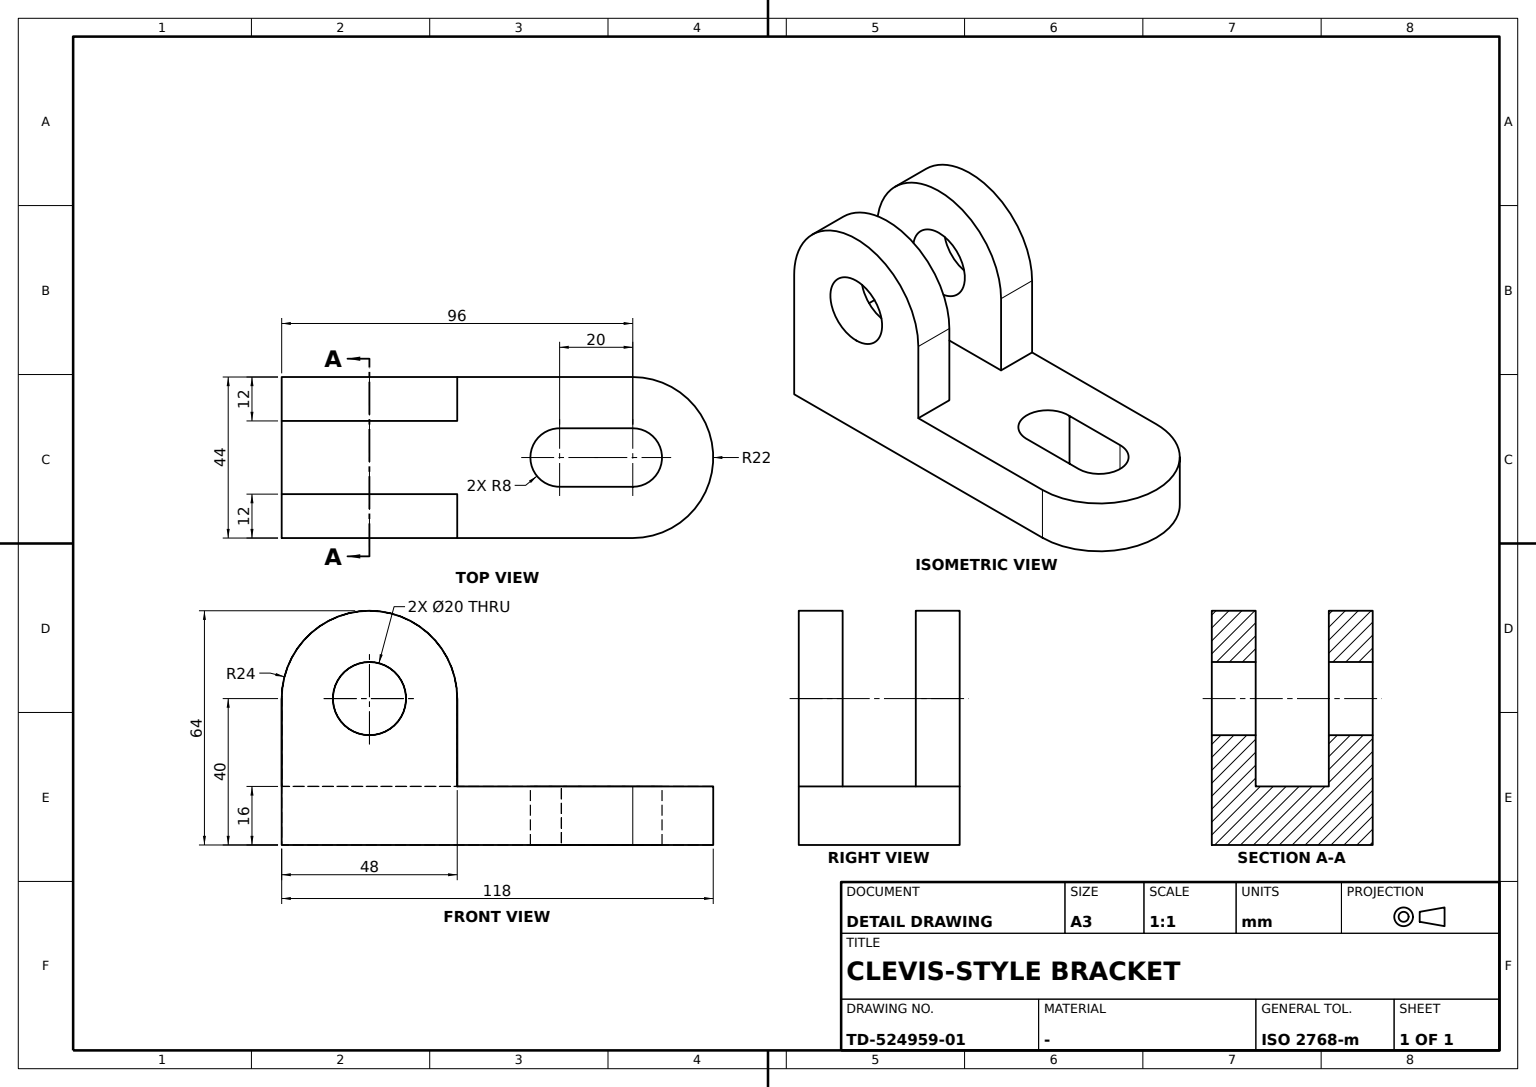
CATIA V5 part; units mm, degrees
sketch "Sketch1" plane through (0, 0, 0) normal (0, 0, 1) x (1, 0, 0)
  line L0 (-48, 22) -> (-48, -22)
  line L1 (-48, -22) -> (48, -22)
  line L2 (48, 22) -> (-48, 22)
  arc A0 (48, -22) -> (48, 22) centre (48, 0) ccw
  arc A1 (48, -8) -> (48, 8) centre (48, 0) ccw
  arc A2 (28.4878, 7.9851) -> (28.4878, -7.9851) centre (28, 0) ccw
  line L3 (28.4878, 7.9851) -> (48, 8)
  point P0 (48, 8)
  line L4 (28.4878, -7.9851) -> (48, -8)
  point P1 (48, -8)
  point P2 (48, 8)
  point P3 (48, -8)
  dimension "length L0" = 44
  dimension "length L1" = 96
  dimension "radius A0" = 22
  dimension "radius A1" = 8
  dimension "radius A2" = 8
  constraint vertical L0 y-axis
  constraint horizontal L1 x-axis
  constraint horizontal L2 x-axis
  constraint symmetry L2 L1 x-axis
  constraint coincidence P0 A1
  constraint coincidence P1 A1
  constraint coincidence P3 P1
  constraint coincidence P2 P0
extrude "Pad1" add sketch "Sketch1" along normal blind 16
sketch "Sketch2" plane through (0, 22, 0) normal (0, 1, 0) x (-1, 0, 0)
  line L0 (0, 16) -> (48, 16)
  line L1 (48, 16) -> (48, 40)
  point P0 (0, 40)
  line L2 (0, 40) -> (0, 16)
  line L3 (-48, 16) -> (48, 16) construction
  line L4 (48, 0) -> (48, 16) construction
  arc A0 (48, 40) -> (0, 40) centre (24, 40) ccw
  circle A1 centre (24, 40) radius 10
  dimension "radius A0" = 24
  dimension "radius A1" = 10
  constraint horizontal L0 x-axis
  constraint vertical L1 y-axis
  constraint vertical L2 y-axis
  constraint coincidence P0 y-axis
  constraint coincidence L0 L3
  constraint coincidence L1 L4
extrude "Pad2" add sketch "Sketch2" against normal blind 12
mirror "Mirror1" about plane through (0, 0, 0) normal (0, 1, 0) of "Pad2"
